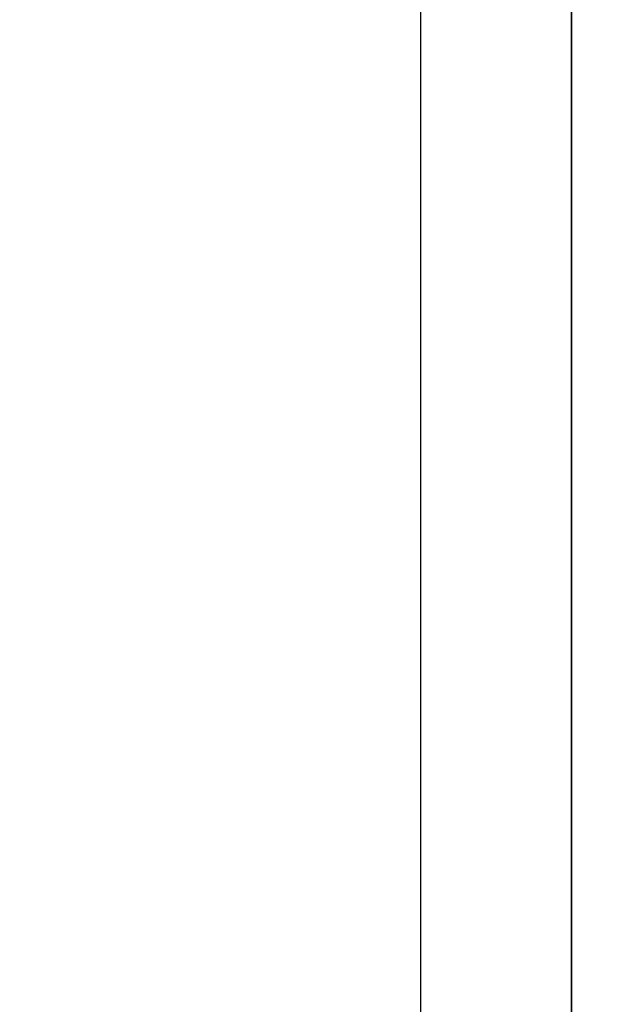
# Model space of a CAD drawing. Units: inches. Extents: x 1291 to 2095, y 532 to 1090.
# Tile 9 of 14: x 1663 to 1696, y 761 to 817. Entities that reach past the tile are written whole.
import ezdxf

# ---------------------------------------------------------------- set-up
doc = ezdxf.new("R2010")
doc.units = ezdxf.units.IN
doc.header["$MEASUREMENT"] = 0
doc.layers.add('A-ANNO-DIMS', color=2, linetype='Continuous', lineweight=18)
doc.layers.add('A-WALL', color=7, linetype='Continuous', lineweight=35)
doc.styles.get("Standard").update_dxf_attribs({"font": 'arial.ttf'})
doc.dimstyles.get("Standard").update_dxf_attribs({"dimtxt": 4, "dimasz": 0.18, "dimexe": 0.18, "dimexo": 0.0625, "dimgap": 0.09, "dimtad": 0, "dimtih": 1, "dimtoh": 1, "dimdec": 0, "dimrnd": 6, "dimzin": 0, "dimdsep": 46, "dimlunit": 3, "dimtxsty": 'Standard', "dimcen": 0.09, "dimadec": 0, "dimazin": 0, "dimtfac": 1, "dimtdec": 0, "dimtofl": 0, "dimtmove": 0, "dimatfit": 3, "dimfxl": 1, "dimtolj": 1, "dimtzin": 0, "dimarcsym": 0})

# ---------------------------------------------------------------- blocks, each defined once
blk = doc.blocks.new('*D46')
at = {"layer": 'A-ANNO-DIMS', "color": 0, "lineweight": -2, "transparency": 16777216}
for p, q in [((1600.27, 579.843), (1600.27, 1087.16)), ((1600.45, 1086.98), (1636.471, 1086.98)), ((1685.404, 1086.98), (1649.383, 1086.98)), ((1685.584, 579.843), (1685.584, 1087.16))]:
    blk.add_line(p, q, dxfattribs=at)
at = {"layer": 'A-ANNO-DIMS', "color": 0, "transparency": 16777216}
for points in [[(1600.45, 1087.01), (1600.45, 1086.95), (1600.27, 1086.98)], [(1685.404, 1087.01), (1685.404, 1086.95), (1685.584, 1086.98)]]:
    blk.add_solid(points, dxfattribs=at)
at = {"layer": 'Defpoints', "color": 0, "transparency": 16777216}
for p in [(1685.584, 1086.98), (1600.27, 579.78), (1685.584, 579.78)]:
    blk.add_point(p, dxfattribs=at)
at = {"layer": 'A-ANNO-DIMS', "color": 0, "transparency": 16777216, "insert": (1642.927, 1086.98), "char_height": 4, "attachment_point": 5}
blk.add_mtext('\\A1;85.31', dxfattribs=at)
blk = doc.blocks.new('*D49')
at = {"layer": 'A-ANNO-DIMS', "color": 0, "lineweight": -2, "transparency": 16777216}
for p, q in [((1694.074, 852.718), (1694.074, 534.4)), ((1586.074, 816.718), (1586.074, 534.4)), ((1586.254, 534.58), (1635.749, 534.58)), ((1693.894, 534.58), (1644.398, 534.58))]:
    blk.add_line(p, q, dxfattribs=at)
at = {"layer": 'A-ANNO-DIMS', "color": 0, "transparency": 16777216}
for points in [[(1586.254, 534.61), (1586.254, 534.55), (1586.074, 534.58)], [(1693.894, 534.61), (1693.894, 534.55), (1694.074, 534.58)]]:
    blk.add_solid(points, dxfattribs=at)
at = {"layer": 'Defpoints', "color": 0, "transparency": 16777216}
for p in [(1694.074, 852.78), (1586.074, 816.78), (1694.074, 534.58)]:
    blk.add_point(p, dxfattribs=at)
at = {"layer": 'A-ANNO-DIMS', "color": 0, "transparency": 16777216, "insert": (1640.074, 534.58), "char_height": 4, "attachment_point": 5}
blk.add_mtext('\\A1;108', dxfattribs=at)
blk = doc.blocks.new('*D51')
at = {"layer": 'A-ANNO-DIMS', "color": 0, "lineweight": -2, "transparency": 16777216}
for p, q in [((1820.011, 852.78), (1297.694, 852.78)), ((1297.874, 852.6), (1297.874, 794.913)), ((1297.874, 732.96), (1297.874, 790.648)), ((1811.011, 732.78), (1297.694, 732.78))]:
    blk.add_line(p, q, dxfattribs=at)
at = {"layer": 'A-ANNO-DIMS', "color": 0, "transparency": 16777216}
for points in [[(1297.844, 852.6), (1297.904, 852.6), (1297.874, 852.78)], [(1297.844, 732.96), (1297.904, 732.96), (1297.874, 732.78)]]:
    blk.add_solid(points, dxfattribs=at)
at = {"layer": 'Defpoints', "color": 0, "transparency": 16777216}
for p in [(1297.874, 852.78), (1820.074, 852.78), (1811.074, 732.78)]:
    blk.add_point(p, dxfattribs=at)
at = {"layer": 'A-ANNO-DIMS', "color": 0, "transparency": 16777216, "insert": (1297.874, 792.78), "char_height": 4, "attachment_point": 5}
blk.add_mtext('\\A1;120', dxfattribs=at)

msp = doc.modelspace()

# ---------------------------------------------------------------- linework, layer by layer
at = {"layer": 'A-WALL'}
msp.add_line((1694.0735, 732.7804), (1694.0735, 852.7804), dxfattribs=at)

# ---------------------------------------------------------------- dimensions: what is measured, and where the dimension line sits
at = {"layer": 'A-ANNO-DIMS'}
for base, p1, p2, override, picture, middle in [((1685.5842, 1086.9804), (1600.2697, 579.7804), (1685.5842, 579.7804), {"dimdec": 2, "dimlfac": 1, "dimrnd": 0, "dimzin": 0, "dimdsep": 46, "dimlunit": 2}, '*D46', (1642.927, 1086.9804)), ((1694.0735, 534.5804), (1586.0735, 816.7804), (1694.0735, 852.7804), {"dimdec": 0, "dimlfac": 1, "dimrnd": 0, "dimzin": 0, "dimdsep": 46, "dimlunit": 2}, '*D49', (1640.0735, 534.5804))]:
    dim = msp.add_linear_dim(base=base, p1=p1, p2=p2, dimstyle='Standard', override=override, dxfattribs=at)
    dim.commit()
    dim.dimension.update_dxf_attribs({"geometry": picture, "text_midpoint": middle})
dim = msp.add_linear_dim(base=(1297.8735, 852.7804), p1=(1811.0735, 732.7804), p2=(1820.0735, 852.7804), angle=90, dimstyle='Standard', override={"dimdec": 0, "dimlfac": 1, "dimrnd": 0, "dimzin": 0, "dimdsep": 46, "dimlunit": 2}, dxfattribs=at)
dim.commit()
dim.dimension.update_dxf_attribs({"geometry": '*D51', "text_midpoint": (1297.8735, 792.7804)})

doc.saveas('drawing.dxf')
